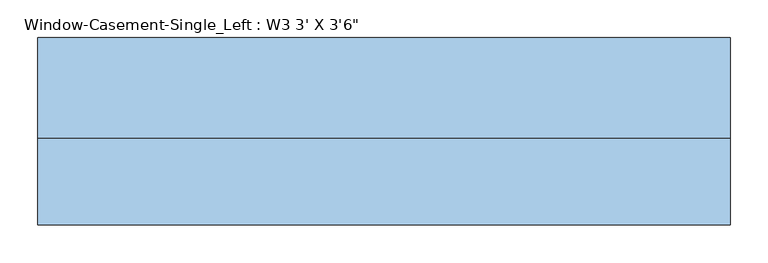
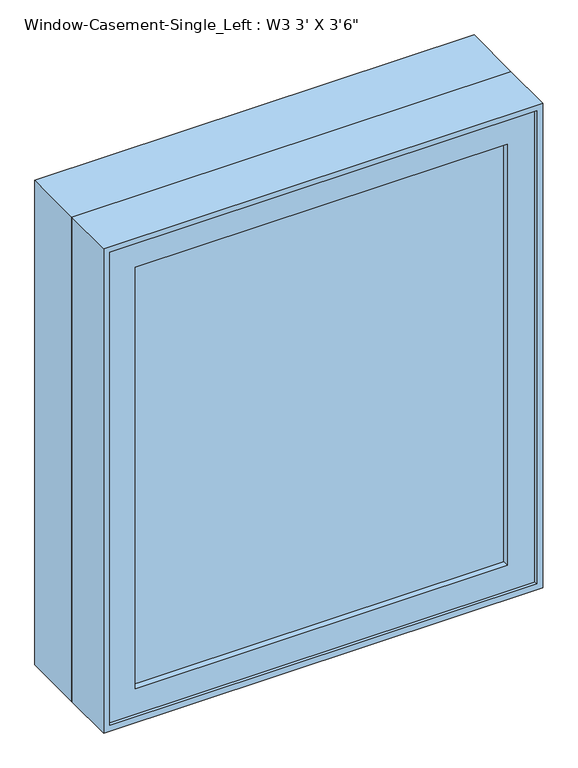
"""IFC4 building model written with IfcOpenShell, lengths in millimetres: window geometry."""

from ifc_helpers import new_model, si_unit, frame, origin, place, context, project, spatial, polyline, outline, extrude, faceted_brep, source, transform, mapped, element, save


def window_cb922c77(model_context):
    return source(origin(), model_context, "Body", "SolidModel", [
        faceted_brep([(425.45, -82.55, 1949.45), (-425.45, -82.55, 1949.45), (-425.45, -19.05, 1949.45), (425.45, -19.05, 1949.45), (444.5, -133.35, 1968.5), (-444.5, -133.35, 1968.5), (-444.5, -82.55, 1968.5), (444.5, -82.55, 1968.5), (457.2, -19.05, 1981.2), (-457.2, -19.05, 1981.2), (-457.2, -133.35, 1981.2), (457.2, -133.35, 1981.2), (-425.45, -82.55, 946.15), (-425.45, -19.05, 946.15), (-444.5, -133.35, 927.1), (-444.5, -82.55, 927.1), (-457.2, -19.05, 914.4), (-457.2, -133.35, 914.4), (425.45, -82.55, 946.15), (425.45, -19.05, 946.15), (444.5, -133.35, 927.1), (444.5, -82.55, 927.1), (457.2, -19.05, 914.4), (457.2, -133.35, 914.4)], [[[0, 1, 2, 3]], [[4, 5, 6, 7]], [[8, 9, 10, 11]], [[1, 12, 13, 2]], [[5, 14, 15, 6]], [[9, 16, 17, 10]], [[12, 18, 19, 13]], [[14, 20, 21, 15]], [[16, 22, 23, 17]], [[9, 8, 22, 16], [3, 2, 13, 19]], [[18, 0, 3, 19]], [[7, 6, 15, 21], [1, 0, 18, 12]], [[20, 4, 7, 21]], [[22, 8, 11, 23]], [[11, 10, 17, 23], [5, 4, 20, 14]]]),
        extrude(outline(polyline([(1981.2, -457.2), (914.4, -457.2), (914.4, 457.2), (1981.2, 457.2), (1981.2, -457.2)]), holes=[polyline([(1962.15, 438.15), (933.45, 438.15), (933.45, -438.15), (1962.15, -438.15), (1962.15, 438.15)])]), frame((0.0, -19.05, 0.0), z_axis=(0.0, 1.0, 0.0), x_axis=(0.0, 0.0, 1.0)), (0.0, 0.0, 1.0), 133.35),
        extrude(outline(polyline([(1968.5, 444.5), (1968.5, -444.5), (927.1, -444.5), (927.1, 444.5), (1968.5, 444.5)]), holes=[polyline([(1911.35, -387.35), (1911.35, 387.35), (984.25, 387.35), (984.25, -387.35), (1911.35, -387.35)])]), frame((0.0, -127.0, 0.0), z_axis=(0.0, 1.0, 0.0), x_axis=(0.0, 0.0, 1.0)), (0.0, 0.0, 1.0), 44.45),
        extrude(outline(polyline([(387.35, -114.3), (-387.35, -114.3), (-387.35, -107.95), (387.35, -107.95), (387.35, -114.3)])), frame((0.0, 0.0, 984.25), z_axis=(0.0, 0.0, 1.0), x_axis=(1.0, 0.0, 0.0)), (0.0, 0.0, 1.0), 927.1),
        extrude(outline(polyline([(-387.35, -95.25), (387.35, -95.25), (387.35, -101.6), (-387.35, -101.6), (-387.35, -95.25)])), frame((0.0, 0.0, 984.25), z_axis=(0.0, 0.0, 1.0), x_axis=(1.0, 0.0, 0.0)), (0.0, 0.0, 1.0), 927.1),
    ])


if __name__ == "__main__":
    model = new_model("IFC4")
    model_context = context("Model", 3, world=origin())
    ifc_project = project(units=[si_unit("LENGTHUNIT", "METRE", prefix="MILLI")], contexts=[model_context])
    site = spatial("IfcSite", under=ifc_project)
    building = spatial("IfcBuilding", under=site)
    placement = place(None, origin())
    window_shape = window_cb922c77(model_context)
    element("IfcWindow", 1, ObjectType="Window-Casement-Single_Left : W3 3' X 3'6\"", at=placement, inside=building, context=model_context, shape_type="MappedRepresentation", body=[
        mapped(window_shape, transform((0.0, 0.0, 0.0), x_axis=(1.0, 0.0, 0.0), y_axis=(0.0, 1.0, 0.0), z_axis=(0.0, 0.0, 1.0))),
    ])
    save(model, "model.ifc")

# Revit data of these elements
# Type "Window-Casement-Single_Left : W3 3' X 3'6\""
#   Type Mark = "20"
#   Fire Rating = "0.5h"
#   Assembly Code = "B2020100"
#   Analytic Construction = "Double glazing - domestic"
#   Window Inset [instance default] = 0' - 0"
#   Wall Thickness [instance default] = 0' - 6"
#   Visual Light Transmittance = 0.81
#   Thermal Resistance (R) = 1.8146 (h·ft²·°F)/BTU
#   Solar Heat Gain Coefficient = 0.76
#   Rough Width = 3' - 0 1/2"
#   Rough Height = 3' - 6 1/2"
#   Interior Wall Closure [instance default] = 0' - 2 1/4"
#   Height = 3' - 6"
#   Heat Transfer Coefficient (U) = 0.5511 BTU/(h·ft²·°F)
#   Frame Extension [instance default] = 0' - 0 1/4"
#   Exterior Wall Closure [instance default] = 0' - 1 1/4"
#   Extension Jamb [instance default] = 0' - 2 1/4"
#   Default Sill Height = 3' - 0"
#   Width = 3' - 0"
#   Muntin Visibility = yes
#   Interior Trim Visibility [instance default] = yes
#   Exterior Trim Visibility [instance default] = yes
#   Extension Jamb Visibility [instance default] = yes
#   Muntin Pattern = Muntin Pattern_2x2 : Muntin Pattern_2x2
#   Interior Trim Material = Wood - Stained
#   Interior Trim = Trim-Window-Interior-Flat : Picture Frame
#   Interior Frame Material = Wood - Stained
#   Glass Panel Material = Glass
#   Exterior Trim Material = Clad - White
#   Exterior Trim = Trim-Window-Exterior-Flat : with Sill
#   Exterior Frame Material = Clad - White
#   Wall Closure = (empty or 0)
# Element 1 (IfcWindow, "Window-Casement-Single_Left : W3 3' X 3'6\"")
#   Wall Thickness = 0' - 9"
#   Extension Jamb = 0' - 5 1/4"
#   Materials on its faces: "Wood - Stained", "Glass", "Clad - White"
# Materials
#   "Wood - Stained": class "Wood", colour RGB 224 178 126, transparency 0, Cost = 0
#   "Glass": class "Glass", colour RGB 0 128 192, transparency 0.75, Description = "Soda Lime Glass", Cost = 0
#   "Clad - White": class "Wood", colour RGB 242 242 238, transparency 0, Cost = 0
